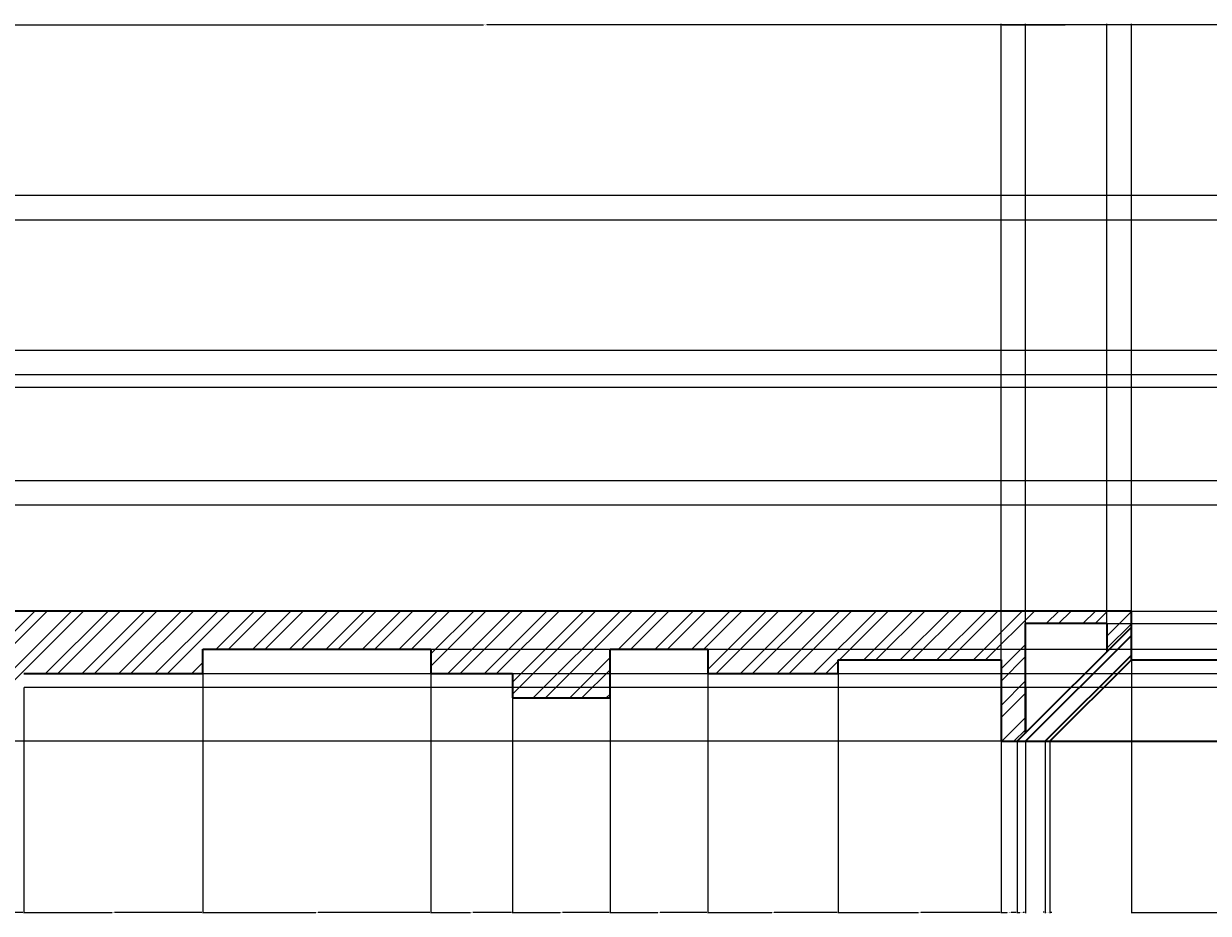
# Model space of a CAD drawing. Units: inches. Extents: x 2121 to 2815, y 1818 to 2233.
# Tile 4 of 6: x 2312 to 2530, y 2070 to 2233. Entities that reach past the tile are written whole.
import ezdxf

# ---------------------------------------------------------------- set-up
doc = ezdxf.new("R2010")
doc.units = ezdxf.units.IN
for name, color, linetype, lineweight in [('A-ANNO-DIMS', 2, 'Continuous', 18), ('A-COLS', 7, 'Continuous', 35), ('A-WALL', 7, 'Continuous', 35), ('A-WALL-PATT', 8, 'Continuous', 13)]:
    doc.layers.add(name, color=color, linetype=linetype, lineweight=lineweight)
doc.styles.get("Standard").update_dxf_attribs({"font": 'arial.ttf'})
doc.dimstyles.get("Standard").update_dxf_attribs({"dimtxt": 0.18, "dimasz": 0.18, "dimexe": 0.18, "dimexo": 0.0625, "dimgap": 0.09, "dimtad": 0, "dimtih": 1, "dimtoh": 1, "dimdec": 4, "dimzin": 0, "dimdsep": 46, "dimtxsty": 'Standard', "dimcen": 0.09, "dimadec": 0, "dimazin": 0, "dimtfac": 1, "dimtdec": 4, "dimtofl": 0, "dimtmove": 0, "dimatfit": 3, "dimfxl": 1, "dimtolj": 1, "dimtzin": 0, "dimarcsym": 0})

# ---------------------------------------------------------------- blocks, each defined once
blk = doc.blocks.new('*D10')
at = {"layer": 'A-ANNO-DIMS', "color": 0, "lineweight": -2, "transparency": 16777216}
for p, q in [((2152.83, 2129.87), (2152.83, 2233.48)), ((2153.01, 2233.3), (2396.54, 2233.3)), ((2640.65, 2233.3), (2397.13, 2233.3)), ((2640.83, 2129.87), (2640.83, 2233.48))]:
    blk.add_line(p, q, dxfattribs=at)
at = {"layer": 'A-ANNO-DIMS', "color": 0, "transparency": 16777216}
for points in [[(2153.01, 2233.33), (2153.01, 2233.27), (2152.83, 2233.3)], [(2640.65, 2233.33), (2640.65, 2233.27), (2640.83, 2233.3)]]:
    blk.add_solid(points, dxfattribs=at)
at = {"layer": 'Defpoints', "color": 0, "transparency": 16777216}
for p in [(2640.83, 2233.3), (2152.83, 2129.81), (2640.83, 2129.81)]:
    blk.add_point(p, dxfattribs=at)
at = {"layer": 'A-ANNO-DIMS', "color": 0, "transparency": 16777216, "insert": (2396.83, 2233.3), "char_height": 0.18, "attachment_point": 5}
blk.add_mtext('\\A1;488', dxfattribs=at)
blk = doc.blocks.new('*D17')
at = {"layer": 'A-ANNO-DIMS', "color": 0, "lineweight": -2, "transparency": 16777216}
for p, q in [((2287.83, 2111.25), (2287.83, 2069.63)), ((2311.83, 2111.25), (2311.83, 2069.63)), ((2288.01, 2069.81), (2299.61, 2069.81)), ((2311.65, 2069.81), (2300.05, 2069.81))]:
    blk.add_line(p, q, dxfattribs=at)
at = {"layer": 'A-ANNO-DIMS', "color": 0, "transparency": 16777216}
for points in [[(2288.01, 2069.84), (2288.01, 2069.78), (2287.83, 2069.81)], [(2311.65, 2069.84), (2311.65, 2069.78), (2311.83, 2069.81)]]:
    blk.add_solid(points, dxfattribs=at)
at = {"layer": 'Defpoints', "color": 0, "transparency": 16777216}
for p in [(2287.83, 2111.31), (2311.83, 2111.31), (2311.83, 2069.81)]:
    blk.add_point(p, dxfattribs=at)
at = {"layer": 'A-ANNO-DIMS', "color": 0, "transparency": 16777216, "insert": (2299.83, 2069.81), "char_height": 0.18, "attachment_point": 5}
blk.add_mtext('\\A1;24', dxfattribs=at)
blk = doc.blocks.new('*D18')
at = {"layer": 'A-ANNO-DIMS', "color": 0, "lineweight": -2, "transparency": 16777216}
for p, q in [((2344.83, 2113.75), (2344.83, 2069.63)), ((2311.83, 2111.25), (2311.83, 2069.63)), ((2312.01, 2069.81), (2328.11, 2069.81)), ((2344.65, 2069.81), (2328.55, 2069.81))]:
    blk.add_line(p, q, dxfattribs=at)
at = {"layer": 'A-ANNO-DIMS', "color": 0, "transparency": 16777216}
for points in [[(2312.01, 2069.84), (2312.01, 2069.78), (2311.83, 2069.81)], [(2344.65, 2069.84), (2344.65, 2069.78), (2344.83, 2069.81)]]:
    blk.add_solid(points, dxfattribs=at)
at = {"layer": 'Defpoints', "color": 0, "transparency": 16777216}
for p in [(2344.83, 2113.81), (2311.83, 2111.31), (2344.83, 2069.81)]:
    blk.add_point(p, dxfattribs=at)
at = {"layer": 'A-ANNO-DIMS', "color": 0, "transparency": 16777216, "insert": (2328.33, 2069.81), "char_height": 0.18, "attachment_point": 5}
blk.add_mtext('\\A1;33', dxfattribs=at)
blk = doc.blocks.new('*D19')
at = {"layer": 'A-ANNO-DIMS', "color": 0, "lineweight": -2, "transparency": 16777216}
for p, q in [((2344.83, 2113.75), (2344.83, 2069.63)), ((2386.83, 2113.75), (2386.83, 2069.63)), ((2345.01, 2069.81), (2365.61, 2069.81)), ((2386.65, 2069.81), (2366.05, 2069.81))]:
    blk.add_line(p, q, dxfattribs=at)
at = {"layer": 'A-ANNO-DIMS', "color": 0, "transparency": 16777216}
for points in [[(2345.01, 2069.84), (2345.01, 2069.78), (2344.83, 2069.81)], [(2386.65, 2069.84), (2386.65, 2069.78), (2386.83, 2069.81)]]:
    blk.add_solid(points, dxfattribs=at)
at = {"layer": 'Defpoints', "color": 0, "transparency": 16777216}
for p in [(2344.83, 2113.81), (2386.83, 2113.81), (2386.83, 2069.81)]:
    blk.add_point(p, dxfattribs=at)
at = {"layer": 'A-ANNO-DIMS', "color": 0, "transparency": 16777216, "insert": (2365.83, 2069.81), "char_height": 0.18, "attachment_point": 5}
blk.add_mtext('\\A1;42', dxfattribs=at)
blk = doc.blocks.new('*D20')
at = {"layer": 'A-ANNO-DIMS', "color": 0, "lineweight": -2, "transparency": 16777216}
for p, q in [((2386.83, 2113.75), (2386.83, 2069.63)), ((2401.83, 2109.25), (2401.83, 2069.63)), ((2387.01, 2069.81), (2394.12, 2069.81)), ((2401.65, 2069.81), (2394.54, 2069.81))]:
    blk.add_line(p, q, dxfattribs=at)
at = {"layer": 'A-ANNO-DIMS', "color": 0, "transparency": 16777216}
for points in [[(2387.01, 2069.84), (2387.01, 2069.78), (2386.83, 2069.81)], [(2401.65, 2069.84), (2401.65, 2069.78), (2401.83, 2069.81)]]:
    blk.add_solid(points, dxfattribs=at)
at = {"layer": 'Defpoints', "color": 0, "transparency": 16777216}
for p in [(2386.83, 2113.81), (2401.83, 2109.31), (2401.83, 2069.81)]:
    blk.add_point(p, dxfattribs=at)
at = {"layer": 'A-ANNO-DIMS', "color": 0, "transparency": 16777216, "insert": (2394.33, 2069.81), "char_height": 0.18, "attachment_point": 5}
blk.add_mtext('\\A1;15', dxfattribs=at)
blk = doc.blocks.new('*D21')
at = {"layer": 'A-ANNO-DIMS', "color": 0, "lineweight": -2, "transparency": 16777216}
for p, q in [((2401.83, 2109.25), (2401.83, 2069.63)), ((2419.83, 2109.25), (2419.83, 2069.63)), ((2402.01, 2069.81), (2410.62, 2069.81)), ((2419.65, 2069.81), (2411.04, 2069.81))]:
    blk.add_line(p, q, dxfattribs=at)
at = {"layer": 'A-ANNO-DIMS', "color": 0, "transparency": 16777216}
for points in [[(2402.01, 2069.84), (2402.01, 2069.78), (2401.83, 2069.81)], [(2419.65, 2069.84), (2419.65, 2069.78), (2419.83, 2069.81)]]:
    blk.add_solid(points, dxfattribs=at)
at = {"layer": 'Defpoints', "color": 0, "transparency": 16777216}
for p in [(2401.83, 2109.31), (2419.83, 2109.31), (2419.83, 2069.81)]:
    blk.add_point(p, dxfattribs=at)
at = {"layer": 'A-ANNO-DIMS', "color": 0, "transparency": 16777216, "insert": (2410.83, 2069.81), "char_height": 0.18, "attachment_point": 5}
blk.add_mtext('\\A1;18', dxfattribs=at)
blk = doc.blocks.new('*D22')
at = {"layer": 'A-ANNO-DIMS', "color": 0, "lineweight": -2, "transparency": 16777216}
for p, q in [((2437.83, 2113.75), (2437.83, 2069.63)), ((2419.83, 2109.25), (2419.83, 2069.63)), ((2420.01, 2069.81), (2428.62, 2069.81)), ((2437.65, 2069.81), (2429.04, 2069.81))]:
    blk.add_line(p, q, dxfattribs=at)
at = {"layer": 'A-ANNO-DIMS', "color": 0, "transparency": 16777216}
for points in [[(2420.01, 2069.84), (2420.01, 2069.78), (2419.83, 2069.81)], [(2437.65, 2069.84), (2437.65, 2069.78), (2437.83, 2069.81)]]:
    blk.add_solid(points, dxfattribs=at)
at = {"layer": 'Defpoints', "color": 0, "transparency": 16777216}
for p in [(2437.83, 2113.81), (2419.83, 2109.31), (2437.83, 2069.81)]:
    blk.add_point(p, dxfattribs=at)
at = {"layer": 'A-ANNO-DIMS', "color": 0, "transparency": 16777216, "insert": (2428.83, 2069.81), "char_height": 0.18, "attachment_point": 5}
blk.add_mtext('\\A1;18', dxfattribs=at)
blk = doc.blocks.new('*D23')
at = {"layer": 'A-ANNO-DIMS', "color": 0, "lineweight": -2, "transparency": 16777216}
for p, q in [((2437.83, 2113.75), (2437.83, 2069.63)), ((2461.83, 2113.75), (2461.83, 2069.63)), ((2438.01, 2069.81), (2449.61, 2069.81)), ((2461.65, 2069.81), (2450.05, 2069.81))]:
    blk.add_line(p, q, dxfattribs=at)
at = {"layer": 'A-ANNO-DIMS', "color": 0, "transparency": 16777216}
for points in [[(2438.01, 2069.84), (2438.01, 2069.78), (2437.83, 2069.81)], [(2461.65, 2069.84), (2461.65, 2069.78), (2461.83, 2069.81)]]:
    blk.add_solid(points, dxfattribs=at)
at = {"layer": 'Defpoints', "color": 0, "transparency": 16777216}
for p in [(2437.83, 2113.81), (2461.83, 2113.81), (2461.83, 2069.81)]:
    blk.add_point(p, dxfattribs=at)
at = {"layer": 'A-ANNO-DIMS', "color": 0, "transparency": 16777216, "insert": (2449.83, 2069.81), "char_height": 0.18, "attachment_point": 5}
blk.add_mtext('\\A1;24', dxfattribs=at)
blk = doc.blocks.new('*D24')
at = {"layer": 'A-ANNO-DIMS', "color": 0, "lineweight": -2, "transparency": 16777216}
for p, q in [((2461.83, 2113.75), (2461.83, 2069.63)), ((2491.83, 2101.25), (2491.83, 2069.63)), ((2462.01, 2069.81), (2476.61, 2069.81)), ((2491.65, 2069.81), (2477.05, 2069.81))]:
    blk.add_line(p, q, dxfattribs=at)
at = {"layer": 'A-ANNO-DIMS', "color": 0, "transparency": 16777216}
for points in [[(2462.01, 2069.84), (2462.01, 2069.78), (2461.83, 2069.81)], [(2491.65, 2069.84), (2491.65, 2069.78), (2491.83, 2069.81)]]:
    blk.add_solid(points, dxfattribs=at)
at = {"layer": 'Defpoints', "color": 0, "transparency": 16777216}
for p in [(2461.83, 2113.81), (2491.83, 2101.31), (2491.83, 2069.81)]:
    blk.add_point(p, dxfattribs=at)
at = {"layer": 'A-ANNO-DIMS', "color": 0, "transparency": 16777216, "insert": (2476.83, 2069.81), "char_height": 0.18, "attachment_point": 5}
blk.add_mtext('\\A1;30', dxfattribs=at)
blk = doc.blocks.new('*D25')
at = {"layer": 'A-ANNO-DIMS', "color": 0, "lineweight": -2, "transparency": 16777216}
for p, q in [((2491.83, 2101.37), (2491.83, 2233.48)), ((2492.01, 2233.3), (2503.61, 2233.3)), ((2515.65, 2233.3), (2504.05, 2233.3)), ((2515.83, 2125.37), (2515.83, 2233.48))]:
    blk.add_line(p, q, dxfattribs=at)
at = {"layer": 'A-ANNO-DIMS', "color": 0, "transparency": 16777216}
for points in [[(2492.01, 2233.33), (2492.01, 2233.27), (2491.83, 2233.3)], [(2515.65, 2233.33), (2515.65, 2233.27), (2515.83, 2233.3)]]:
    blk.add_solid(points, dxfattribs=at)
at = {"layer": 'Defpoints', "color": 0, "transparency": 16777216}
for p in [(2515.83, 2233.3), (2515.83, 2125.31), (2491.83, 2101.31)]:
    blk.add_point(p, dxfattribs=at)
at = {"layer": 'A-ANNO-DIMS', "color": 0, "transparency": 16777216, "insert": (2503.83, 2233.3), "char_height": 0.18, "attachment_point": 5}
blk.add_mtext('\\A1;24', dxfattribs=at)
blk = doc.blocks.new('*D26')
at = {"layer": 'A-ANNO-DIMS', "color": 0, "lineweight": -2, "transparency": 16777216}
for p, q in [((2515.83, 2116.25), (2515.83, 2069.63)), ((2619.83, 2108.3), (2619.83, 2069.63)), ((2516.01, 2069.81), (2567.55, 2069.81)), ((2619.65, 2069.81), (2568.11, 2069.81))]:
    blk.add_line(p, q, dxfattribs=at)
at = {"layer": 'A-ANNO-DIMS', "color": 0, "transparency": 16777216}
for points in [[(2516.01, 2069.84), (2516.01, 2069.78), (2515.83, 2069.81)], [(2619.65, 2069.84), (2619.65, 2069.78), (2619.83, 2069.81)]]:
    blk.add_solid(points, dxfattribs=at)
at = {"layer": 'Defpoints', "color": 0, "transparency": 16777216}
for p in [(2515.83, 2116.31), (2619.83, 2108.36), (2619.83, 2069.81)]:
    blk.add_point(p, dxfattribs=at)
at = {"layer": 'A-ANNO-DIMS', "color": 0, "transparency": 16777216, "insert": (2567.83, 2069.81), "char_height": 0.18, "attachment_point": 5}
blk.add_mtext('\\A1;104', dxfattribs=at)
blk = doc.blocks.new('*D32')
at = {"layer": 'A-ANNO-DIMS', "color": 0, "lineweight": -2, "transparency": 16777216}
for p, q in [((2311.9, 2113.81), (2814.07, 2113.81)), ((2813.89, 2113.63), (2813.89, 2112.74)), ((2813.89, 2111.49), (2813.89, 2112.38)), ((2311.9, 2111.31), (2814.07, 2111.31))]:
    blk.add_line(p, q, dxfattribs=at)
at = {"layer": 'A-ANNO-DIMS', "color": 0, "transparency": 16777216}
for points in [[(2813.86, 2113.63), (2813.92, 2113.63), (2813.89, 2113.81)], [(2813.86, 2111.49), (2813.92, 2111.49), (2813.89, 2111.31)]]:
    blk.add_solid(points, dxfattribs=at)
at = {"layer": 'Defpoints', "color": 0, "transparency": 16777216}
for p in [(2311.83, 2113.81), (2311.83, 2111.31), (2813.89, 2111.31)]:
    blk.add_point(p, dxfattribs=at)
at = {"layer": 'A-ANNO-DIMS', "color": 0, "transparency": 16777216, "insert": (2813.89, 2112.56), "char_height": 0.18, "attachment_point": 5}
blk.add_mtext('\\A1;2.5', dxfattribs=at)
blk = doc.blocks.new('*D33')
at = {"layer": 'A-ANNO-DIMS', "color": 0, "lineweight": -2, "transparency": 16777216}
for p, q in [((2386.9, 2118.31), (2814.07, 2118.31)), ((2813.89, 2118.13), (2813.89, 2116.24)), ((2813.89, 2113.99), (2813.89, 2115.88)), ((2386.9, 2113.81), (2814.07, 2113.81))]:
    blk.add_line(p, q, dxfattribs=at)
at = {"layer": 'A-ANNO-DIMS', "color": 0, "transparency": 16777216}
for points in [[(2813.86, 2118.13), (2813.92, 2118.13), (2813.89, 2118.31)], [(2813.86, 2113.99), (2813.92, 2113.99), (2813.89, 2113.81)]]:
    blk.add_solid(points, dxfattribs=at)
at = {"layer": 'Defpoints', "color": 0, "transparency": 16777216}
for p in [(2386.83, 2118.31), (2386.83, 2113.81), (2813.89, 2113.81)]:
    blk.add_point(p, dxfattribs=at)
at = {"layer": 'A-ANNO-DIMS', "color": 0, "transparency": 16777216, "insert": (2813.89, 2116.06), "char_height": 0.18, "attachment_point": 5}
blk.add_mtext('\\A1;4.5', dxfattribs=at)
blk = doc.blocks.new('*D34')
at = {"layer": 'A-ANNO-DIMS', "color": 0, "lineweight": -2, "transparency": 16777216}
for p, q in [((2515.9, 2116.31), (2814.07, 2116.31)), ((2813.89, 2116.13), (2813.89, 2108.99)), ((2813.89, 2101.49), (2813.89, 2108.63)), ((2500.9, 2101.31), (2814.07, 2101.31))]:
    blk.add_line(p, q, dxfattribs=at)
at = {"layer": 'A-ANNO-DIMS', "color": 0, "transparency": 16777216}
for points in [[(2813.86, 2116.13), (2813.92, 2116.13), (2813.89, 2116.31)], [(2813.86, 2101.49), (2813.92, 2101.49), (2813.89, 2101.31)]]:
    blk.add_solid(points, dxfattribs=at)
at = {"layer": 'Defpoints', "color": 0, "transparency": 16777216}
for p in [(2515.83, 2116.31), (2500.83, 2101.31), (2813.89, 2101.31)]:
    blk.add_point(p, dxfattribs=at)
at = {"layer": 'A-ANNO-DIMS', "color": 0, "transparency": 16777216, "insert": (2813.89, 2108.81), "char_height": 0.18, "attachment_point": 5}
blk.add_mtext('\\A1;15', dxfattribs=at)
blk = doc.blocks.new('*D36')
at = {"layer": 'A-ANNO-DIMS', "color": 0, "lineweight": -2, "transparency": 16777216}
for p, q in [((2515.77, 2125.31), (2121.16, 2125.31)), ((2121.34, 2125.13), (2121.34, 2113.49)), ((2121.34, 2101.49), (2121.34, 2113.13)), ((2491.77, 2101.31), (2121.16, 2101.31))]:
    blk.add_line(p, q, dxfattribs=at)
at = {"layer": 'A-ANNO-DIMS', "color": 0, "transparency": 16777216}
for points in [[(2121.31, 2125.13), (2121.37, 2125.13), (2121.34, 2125.31)], [(2121.31, 2101.49), (2121.37, 2101.49), (2121.34, 2101.31)]]:
    blk.add_solid(points, dxfattribs=at)
at = {"layer": 'Defpoints', "color": 0, "transparency": 16777216}
for p in [(2121.34, 2125.31), (2515.83, 2125.31), (2491.83, 2101.31)]:
    blk.add_point(p, dxfattribs=at)
at = {"layer": 'A-ANNO-DIMS', "color": 0, "transparency": 16777216, "insert": (2121.34, 2113.31), "char_height": 0.18, "attachment_point": 5}
blk.add_mtext('\\A1;24', dxfattribs=at)
blk = doc.blocks.new('*D37')
at = {"layer": 'A-ANNO-DIMS', "color": 0, "lineweight": -2, "transparency": 16777216}
for p, q in [((2491.83, 2116.37), (2491.83, 2233.48)), ((2492.01, 2233.3), (2493.82, 2233.3)), ((2496.15, 2233.3), (2494.34, 2233.3)), ((2496.33, 2123.06), (2496.33, 2233.48))]:
    blk.add_line(p, q, dxfattribs=at)
at = {"layer": 'A-ANNO-DIMS', "color": 0, "transparency": 16777216}
for points in [[(2492.01, 2233.33), (2492.01, 2233.27), (2491.83, 2233.3)], [(2496.15, 2233.33), (2496.15, 2233.27), (2496.33, 2233.3)]]:
    blk.add_solid(points, dxfattribs=at)
at = {"layer": 'Defpoints', "color": 0, "transparency": 16777216}
for p in [(2496.33, 2233.3), (2496.33, 2122.99), (2491.83, 2116.31)]:
    blk.add_point(p, dxfattribs=at)
at = {"layer": 'A-ANNO-DIMS', "color": 0, "transparency": 16777216, "insert": (2494.08, 2233.3), "char_height": 0.18, "attachment_point": 5}
blk.add_mtext('\\A1;4.5', dxfattribs=at)
blk = doc.blocks.new('*D38')
at = {"layer": 'A-ANNO-DIMS', "color": 0, "lineweight": -2, "transparency": 16777216}
for p, q in [((2496.33, 2123.06), (2496.33, 2233.48)), ((2496.51, 2233.3), (2503.62, 2233.3)), ((2511.15, 2233.3), (2504.04, 2233.3)), ((2511.33, 2123.06), (2511.33, 2233.48))]:
    blk.add_line(p, q, dxfattribs=at)
at = {"layer": 'A-ANNO-DIMS', "color": 0, "transparency": 16777216}
for points in [[(2496.51, 2233.33), (2496.51, 2233.27), (2496.33, 2233.3)], [(2511.15, 2233.33), (2511.15, 2233.27), (2511.33, 2233.3)]]:
    blk.add_solid(points, dxfattribs=at)
at = {"layer": 'Defpoints', "color": 0, "transparency": 16777216}
for p in [(2511.33, 2233.3), (2496.33, 2122.99), (2511.33, 2122.99)]:
    blk.add_point(p, dxfattribs=at)
at = {"layer": 'A-ANNO-DIMS', "color": 0, "transparency": 16777216, "insert": (2503.83, 2233.3), "char_height": 0.18, "attachment_point": 5}
blk.add_mtext('\\A1;15', dxfattribs=at)
blk = doc.blocks.new('*D39')
at = {"layer": 'A-ANNO-DIMS', "color": 0, "lineweight": -2, "transparency": 16777216}
for p, q in [((2515.9, 2125.31), (2814.07, 2125.31)), ((2813.89, 2125.13), (2813.89, 2124.33)), ((2511.4, 2122.99), (2814.07, 2122.99)), ((2813.89, 2123.17), (2813.89, 2123.97))]:
    blk.add_line(p, q, dxfattribs=at)
at = {"layer": 'A-ANNO-DIMS', "color": 0, "transparency": 16777216}
for points in [[(2813.86, 2125.13), (2813.92, 2125.13), (2813.89, 2125.31)], [(2813.86, 2123.17), (2813.92, 2123.17), (2813.89, 2122.99)]]:
    blk.add_solid(points, dxfattribs=at)
at = {"layer": 'Defpoints', "color": 0, "transparency": 16777216}
for p in [(2515.83, 2125.31), (2813.89, 2125.31), (2511.33, 2122.99)]:
    blk.add_point(p, dxfattribs=at)
at = {"layer": 'A-ANNO-DIMS', "color": 0, "transparency": 16777216, "insert": (2813.89, 2124.15), "char_height": 0.18, "attachment_point": 5}
blk.add_mtext('\\A1;2.314', dxfattribs=at)
blk = doc.blocks.new('*D40')
at = {"layer": 'A-ANNO-DIMS', "color": 0, "lineweight": -2, "transparency": 16777216}
for p, q in [((2491.83, 2101.25), (2491.83, 2069.63)), ((2494.81, 2101.25), (2494.81, 2069.63)), ((2492.01, 2069.81), (2492.95, 2069.81)), ((2494.63, 2069.81), (2493.7, 2069.81))]:
    blk.add_line(p, q, dxfattribs=at)
at = {"layer": 'A-ANNO-DIMS', "color": 0, "transparency": 16777216}
for points in [[(2492.01, 2069.84), (2492.01, 2069.78), (2491.83, 2069.81)], [(2494.63, 2069.84), (2494.63, 2069.78), (2494.81, 2069.81)]]:
    blk.add_solid(points, dxfattribs=at)
at = {"layer": 'Defpoints', "color": 0, "transparency": 16777216}
for p in [(2491.83, 2101.31), (2494.81, 2101.31), (2494.81, 2069.81)]:
    blk.add_point(p, dxfattribs=at)
at = {"layer": 'A-ANNO-DIMS', "color": 0, "transparency": 16777216, "insert": (2493.32, 2069.81), "char_height": 0.18, "attachment_point": 5}
blk.add_mtext('\\A1;2.981', dxfattribs=at)
blk = doc.blocks.new('*D41')
at = {"layer": 'A-ANNO-DIMS', "color": 0, "lineweight": -2, "transparency": 16777216}
for p, q in [((2494.81, 2101.25), (2494.81, 2069.63)), ((2496.33, 2101.25), (2496.33, 2069.63)), ((2494.99, 2069.81), (2495.26, 2069.81)), ((2496.15, 2069.81), (2495.89, 2069.81))]:
    blk.add_line(p, q, dxfattribs=at)
at = {"layer": 'A-ANNO-DIMS', "color": 0, "transparency": 16777216}
for points in [[(2494.99, 2069.84), (2494.99, 2069.78), (2494.81, 2069.81)], [(2496.15, 2069.84), (2496.15, 2069.78), (2496.33, 2069.81)]]:
    blk.add_solid(points, dxfattribs=at)
at = {"layer": 'Defpoints', "color": 0, "transparency": 16777216}
for p in [(2494.81, 2101.31), (2496.33, 2101.31), (2496.33, 2069.81)]:
    blk.add_point(p, dxfattribs=at)
at = {"layer": 'A-ANNO-DIMS', "color": 0, "transparency": 16777216, "insert": (2495.57, 2069.81), "char_height": 0.18, "attachment_point": 5}
blk.add_mtext('\\A1;1.52', dxfattribs=at)
blk = doc.blocks.new('*D42')
at = {"layer": 'A-ANNO-DIMS', "color": 0, "lineweight": -2, "transparency": 16777216}
for p, q in [((2499.935347, 2101.246525), (2499.935347, 2069.634025)), ((2500.832641, 2101.246525), (2500.832641, 2069.634025)), ((2499.755347, 2069.814025), (2499.575347, 2069.814025)), ((2501.012641, 2069.814025), (2501.192641, 2069.814025))]:
    blk.add_line(p, q, dxfattribs=at)
at = {"layer": 'A-ANNO-DIMS', "color": 0, "transparency": 16777216}
for points in [[(2499.755347, 2069.844025), (2499.755347, 2069.784025), (2499.935347, 2069.814025)], [(2501.012641, 2069.844025), (2501.012641, 2069.784025), (2500.832641, 2069.814025)]]:
    blk.add_solid(points, dxfattribs=at)
at = {"layer": 'Defpoints', "color": 0, "transparency": 16777216}
for p in [(2499.935347, 2101.309025), (2500.832641, 2101.309025), (2500.832641, 2069.814025)]:
    blk.add_point(p, dxfattribs=at)
at = {"layer": 'A-ANNO-DIMS', "color": 0, "transparency": 16777216, "insert": (2500.383994, 2069.814025), "char_height": 0.18, "attachment_point": 5}
blk.add_mtext('\\A1;0.90', dxfattribs=at)
blk = doc.blocks.new('*D86')
at = {"layer": 'A-ANNO-DIMS', "color": 0, "lineweight": -2, "transparency": 16777216}
for p, q in [((2760.77, 2144.81), (2121.16, 2144.81)), ((2121.34, 2144.63), (2121.34, 2123.24)), ((2121.34, 2101.49), (2121.34, 2122.88)), ((2760.77, 2101.31), (2121.16, 2101.31))]:
    blk.add_line(p, q, dxfattribs=at)
at = {"layer": 'A-ANNO-DIMS', "color": 0, "transparency": 16777216}
for points in [[(2121.31, 2144.63), (2121.37, 2144.63), (2121.34, 2144.81)], [(2121.31, 2101.49), (2121.37, 2101.49), (2121.34, 2101.31)]]:
    blk.add_solid(points, dxfattribs=at)
at = {"layer": 'Defpoints', "color": 0, "transparency": 16777216}
for p in [(2121.34, 2144.81), (2760.83, 2144.81), (2760.83, 2101.31)]:
    blk.add_point(p, dxfattribs=at)
at = {"layer": 'A-ANNO-DIMS', "color": 0, "transparency": 16777216, "insert": (2121.34, 2123.06), "char_height": 0.18, "attachment_point": 5}
blk.add_mtext('\\A1;43.5', dxfattribs=at)
blk = doc.blocks.new('*D88')
at = {"layer": 'A-ANNO-DIMS', "color": 0, "lineweight": -2, "transparency": 16777216}
for p, q in [((2760.77, 2197.31), (2121.16, 2197.31)), ((2121.34, 2197.13), (2121.34, 2185.49)), ((2121.34, 2173.49), (2121.34, 2185.13)), ((2760.77, 2173.31), (2121.16, 2173.31))]:
    blk.add_line(p, q, dxfattribs=at)
at = {"layer": 'A-ANNO-DIMS', "color": 0, "transparency": 16777216}
for points in [[(2121.31, 2197.13), (2121.37, 2197.13), (2121.34, 2197.31)], [(2121.31, 2173.49), (2121.37, 2173.49), (2121.34, 2173.31)]]:
    blk.add_solid(points, dxfattribs=at)
at = {"layer": 'Defpoints', "color": 0, "transparency": 16777216}
for p in [(2121.34, 2197.31), (2760.83, 2197.31), (2760.83, 2173.31)]:
    blk.add_point(p, dxfattribs=at)
at = {"layer": 'A-ANNO-DIMS', "color": 0, "transparency": 16777216, "insert": (2121.34, 2185.31), "char_height": 0.18, "attachment_point": 5}
blk.add_mtext('\\A1;24', dxfattribs=at)
blk = doc.blocks.new('*D89')
at = {"layer": 'A-ANNO-DIMS', "color": 0, "lineweight": -2, "transparency": 16777216}
for p, q in [((2756.07, 2201.81), (2121.16, 2201.81)), ((2121.34, 2201.63), (2121.34, 2199.74)), ((2121.34, 2197.49), (2121.34, 2199.38)), ((2760.77, 2197.31), (2121.16, 2197.31))]:
    blk.add_line(p, q, dxfattribs=at)
at = {"layer": 'A-ANNO-DIMS', "color": 0, "transparency": 16777216}
for points in [[(2121.31, 2201.63), (2121.37, 2201.63), (2121.34, 2201.81)], [(2121.31, 2197.49), (2121.37, 2197.49), (2121.34, 2197.31)]]:
    blk.add_solid(points, dxfattribs=at)
at = {"layer": 'Defpoints', "color": 0, "transparency": 16777216}
for p in [(2121.34, 2201.81), (2756.14, 2201.81), (2760.83, 2197.31)]:
    blk.add_point(p, dxfattribs=at)
at = {"layer": 'A-ANNO-DIMS', "color": 0, "transparency": 16777216, "insert": (2121.34, 2199.56), "char_height": 0.18, "attachment_point": 5}
blk.add_mtext('\\A1;4.5', dxfattribs=at)
blk = doc.blocks.new('*D90')
at = {"layer": 'A-ANNO-DIMS', "color": 0, "lineweight": -2, "transparency": 16777216}
for p, q in [((2760.77, 2168.81), (2121.16, 2168.81)), ((2121.34, 2168.63), (2121.34, 2159.24)), ((2121.34, 2149.49), (2121.34, 2158.88)), ((2760.77, 2149.31), (2121.16, 2149.31))]:
    blk.add_line(p, q, dxfattribs=at)
at = {"layer": 'A-ANNO-DIMS', "color": 0, "transparency": 16777216}
for points in [[(2121.31, 2168.63), (2121.37, 2168.63), (2121.34, 2168.81)], [(2121.31, 2149.49), (2121.37, 2149.49), (2121.34, 2149.31)]]:
    blk.add_solid(points, dxfattribs=at)
at = {"layer": 'Defpoints', "color": 0, "transparency": 16777216}
for p in [(2121.34, 2168.81), (2760.83, 2168.81), (2760.83, 2149.31)]:
    blk.add_point(p, dxfattribs=at)
at = {"layer": 'A-ANNO-DIMS', "color": 0, "transparency": 16777216, "insert": (2121.34, 2159.06), "char_height": 0.18, "attachment_point": 5}
blk.add_mtext('\\A1;19.5', dxfattribs=at)
blk = doc.blocks.new('*D91')
at = {"layer": 'A-ANNO-DIMS', "color": 0, "lineweight": -2, "transparency": 16777216}
for p, q in [((2760.77, 2149.31), (2121.16, 2149.31)), ((2121.34, 2149.13), (2121.34, 2147.24)), ((2121.34, 2144.99), (2121.34, 2146.88)), ((2760.77, 2144.81), (2121.16, 2144.81))]:
    blk.add_line(p, q, dxfattribs=at)
at = {"layer": 'A-ANNO-DIMS', "color": 0, "transparency": 16777216}
for points in [[(2121.31, 2149.13), (2121.37, 2149.13), (2121.34, 2149.31)], [(2121.31, 2144.99), (2121.37, 2144.99), (2121.34, 2144.81)]]:
    blk.add_solid(points, dxfattribs=at)
at = {"layer": 'Defpoints', "color": 0, "transparency": 16777216}
for p in [(2121.34, 2149.31), (2760.83, 2149.31), (2760.83, 2144.81)]:
    blk.add_point(p, dxfattribs=at)
at = {"layer": 'A-ANNO-DIMS', "color": 0, "transparency": 16777216, "insert": (2121.34, 2147.06), "char_height": 0.18, "attachment_point": 5}
blk.add_mtext('\\A1;4.5', dxfattribs=at)
blk = doc.blocks.new('*D97')
at = {"layer": 'A-ANNO-DIMS', "color": 0, "lineweight": -2, "transparency": 16777216}
for p, q in [((2765.42, 2168.81), (2121.16, 2168.81)), ((2121.34, 2168.63), (2121.34, 2167.83)), ((2765.42, 2166.48), (2121.16, 2166.48)), ((2121.34, 2166.66), (2121.34, 2167.46))]:
    blk.add_line(p, q, dxfattribs=at)
at = {"layer": 'A-ANNO-DIMS', "color": 0, "transparency": 16777216}
for points in [[(2121.31, 2168.63), (2121.37, 2168.63), (2121.34, 2168.81)], [(2121.31, 2166.66), (2121.37, 2166.66), (2121.34, 2166.48)]]:
    blk.add_solid(points, dxfattribs=at)
at = {"layer": 'Defpoints', "color": 0, "transparency": 16777216}
for p in [(2121.34, 2168.81), (2765.49, 2168.81), (2765.49, 2166.48)]:
    blk.add_point(p, dxfattribs=at)
at = {"layer": 'A-ANNO-DIMS', "color": 0, "transparency": 16777216, "insert": (2121.34, 2167.64), "char_height": 0.18, "attachment_point": 5}
blk.add_mtext('\\A1;2.33', dxfattribs=at)

msp = doc.modelspace()

# ---------------------------------------------------------------- hatches: boundary and pattern name
at = {"layer": 'A-WALL-PATT'}
h = msp.add_hatch(dxfattribs=at)
h.set_pattern_fill('ANSI32', color=256, scale=0.5)
h.paths.add_polyline_path([(2496.3326, 2122.9949), (2511.3326, 2122.9949), (2511.3326, 2117.8278), (2515.8326, 2122.3278), (2515.8326, 2125.309), (2157.3326, 2125.309), (2157.3326, 2129.809), (2152.8326, 2129.809), (2152.8326, 2125.309), (2152.8326, 2113.809), (2182.8326, 2113.809), (2182.8326, 2109.309), (2224.8326, 2109.309), (2224.8326, 2113.809), (2260.8326, 2113.809), (2260.8326, 2109.309), (2269.8326, 2109.309), (2269.8326, 2113.809), (2287.8326, 2113.809), (2287.8326, 2111.309), (2311.8326, 2111.309), (2311.8326, 2113.809), (2344.8326, 2113.809), (2344.8326, 2118.309), (2386.8326, 2118.309), (2386.8326, 2113.809), (2401.8326, 2113.809), (2401.8326, 2109.309), (2419.8326, 2109.309), (2419.8326, 2118.309), (2437.8326, 2118.309), (2437.8326, 2113.809), (2461.8326, 2113.809), (2461.8326, 2116.309), (2491.8326, 2116.309), (2491.8326, 2101.309), (2494.8138, 2101.309), (2496.3326, 2102.8278)])
h.paths.add_polyline_path([(2640.8326, 2129.809), (2628.8326, 2129.809), (2628.8326, 2125.309), (2619.8326, 2125.309), (2619.8326, 2108.3582), (2628.8326, 2101.309), (2640.8326, 2101.309)])

# ---------------------------------------------------------------- linework, layer by layer
at = {"layer": 'A-COLS'}
for p, q in [((2515.8326, 2116.309), (2515.8326, 2125.309)), ((2496.3326, 2102.8278), (2496.3326, 2122.9949)), ((2511.3326, 2122.9949), (2496.3326, 2122.9949)), ((2511.3326, 2122.9949), (2511.3326, 2117.8278)), ((2515.8326, 2122.3278), (2494.8138, 2101.309)), ((2515.8326, 2120.809), (2496.3326, 2101.309)), ((2515.8326, 2120.809), (2496.3326, 2101.309)), ((2491.8326, 2116.309), (2491.8326, 2101.309)), ((2515.8326, 2117.2063), (2499.9353, 2101.309)), ((2515.8326, 2116.309), (2500.8326, 2101.309)), ((2496.3326, 2111.2363), (2496.3326, 2111.2363)), ((2496.3326, 2111.2363), (2496.3326, 2102.8278)), ((2491.8326, 2101.309), (2500.8326, 2101.309))]:
    msp.add_line(p, q, dxfattribs=at)
at = {"layer": 'A-WALL'}
for p, q in [((2515.8326, 2125.309), (2157.3326, 2125.309)), ((2344.8326, 2113.809), (2344.8326, 2118.309)), ((2344.8326, 2118.309), (2386.8326, 2118.309)), ((2386.8326, 2118.309), (2386.8326, 2113.809)), ((2419.8326, 2109.309), (2419.8326, 2118.309)), ((2419.8326, 2118.309), (2437.8326, 2118.309)), ((2437.8326, 2118.309), (2437.8326, 2113.809)), ((2461.8326, 2113.809), (2461.8326, 2116.309)), ((2461.8326, 2116.309), (2491.8326, 2116.309)), ((2515.8326, 2116.309), (2619.8326, 2116.309)), ((2311.8326, 2113.809), (2344.8326, 2113.809)), ((2386.8326, 2113.809), (2401.8326, 2113.809)), ((2401.8326, 2113.809), (2401.8326, 2109.309)), ((2437.8326, 2113.809), (2461.8326, 2113.809)), ((2401.8326, 2109.309), (2419.8326, 2109.309)), ((2500.8326, 2101.309), (2778.8326, 2101.309))]:
    msp.add_line(p, q, dxfattribs=at)

# ---------------------------------------------------------------- dimensions: what is measured, and where the dimension line sits
at = {"layer": 'A-ANNO-DIMS'}
for base, p1, p2, override, picture, middle in [((2640.8326, 2233.304), (2152.8326, 2129.809), (2640.8326, 2129.809), {"dimdec": 0, "dimlfac": 1, "dimrnd": 0, "dimzin": 0, "dimdsep": 46, "dimlunit": 2}, '*D10', (2396.8326, 2233.304)), ((2515.8326, 2233.304), (2491.8326, 2101.309), (2515.8326, 2125.309), {"dimdec": 0, "dimlfac": 1, "dimrnd": 0, "dimzin": 0, "dimdsep": 46, "dimlunit": 2}, '*D25', (2503.8326, 2233.304)), ((2496.3326, 2233.304), (2491.8326, 2116.309), (2496.3326, 2122.9949), {"dimdec": 1, "dimlfac": 1, "dimrnd": 0, "dimzin": 0, "dimdsep": 46, "dimlunit": 2}, '*D37', (2494.0826, 2233.304)), ((2511.3326, 2233.304), (2496.3326, 2122.9949), (2511.3326, 2122.9949), {"dimdec": 0, "dimlfac": 1, "dimrnd": 0, "dimzin": 0, "dimdsep": 46, "dimlunit": 2}, '*D38', (2503.8326, 2233.304)), ((2619.8326, 2069.814), (2515.8326, 2116.309), (2619.8326, 2108.3582), {"dimdec": 0, "dimlfac": 1, "dimrnd": 0, "dimzin": 0, "dimdsep": 46, "dimlunit": 2}, '*D26', (2567.8326, 2069.814)), ((2344.8326, 2069.814), (2311.8326, 2111.309), (2344.8326, 2113.809), {"dimdec": 0, "dimlfac": 1, "dimrnd": 0, "dimzin": 0, "dimdsep": 46, "dimlunit": 2}, '*D18', (2328.3326, 2069.814)), ((2386.8326, 2069.814), (2344.8326, 2113.809), (2386.8326, 2113.809), {"dimdec": 0, "dimlfac": 1, "dimrnd": 0, "dimzin": 0, "dimdsep": 46, "dimlunit": 2}, '*D19', (2365.8326, 2069.814)), ((2401.8326, 2069.814), (2386.8326, 2113.809), (2401.8326, 2109.309), {"dimdec": 0, "dimlfac": 1, "dimrnd": 0, "dimzin": 0, "dimdsep": 46, "dimlunit": 2}, '*D20', (2394.3326, 2069.814)), ((2437.8326, 2069.814), (2419.8326, 2109.309), (2437.8326, 2113.809), {"dimdec": 0, "dimlfac": 1, "dimrnd": 0, "dimzin": 0, "dimdsep": 46, "dimlunit": 2}, '*D22', (2428.8326, 2069.814)), ((2461.8326, 2069.814), (2437.8326, 2113.809), (2461.8326, 2113.809), {"dimdec": 0, "dimlfac": 1, "dimrnd": 0, "dimzin": 0, "dimdsep": 46, "dimlunit": 2}, '*D23', (2449.8326, 2069.814)), ((2491.8326, 2069.814), (2461.8326, 2113.809), (2491.8326, 2101.309), {"dimdec": 0, "dimlfac": 1, "dimrnd": 0, "dimzin": 0, "dimdsep": 46, "dimlunit": 2}, '*D24', (2476.8326, 2069.814)), ((2311.8326, 2069.814), (2287.8326, 2111.309), (2311.8326, 2111.309), {"dimdec": 0, "dimlfac": 1, "dimrnd": 0, "dimzin": 0, "dimdsep": 46, "dimlunit": 2}, '*D17', (2299.8326, 2069.814)), ((2419.8326, 2069.814), (2401.8326, 2109.309), (2419.8326, 2109.309), {"dimdec": 0, "dimlfac": 1, "dimrnd": 0, "dimzin": 0, "dimdsep": 46, "dimlunit": 2}, '*D21', (2410.8326, 2069.814)), ((2494.8138, 2069.814), (2491.8326, 2101.309), (2494.8138, 2101.309), {"dimdec": 3, "dimlfac": 1, "dimrnd": 0, "dimzin": 0, "dimdsep": 46, "dimlunit": 2}, '*D40', (2493.3232, 2069.814)), ((2496.3326, 2069.814), (2494.8138, 2101.309), (2496.3326, 2101.309), {"dimdec": 2, "dimlfac": 1, "dimrnd": 0, "dimzin": 0, "dimdsep": 46, "dimlunit": 2}, '*D41', (2495.5732, 2069.814)), ((2500.8326, 2069.814), (2499.9353, 2101.309), (2500.8326, 2101.309), {"dimdec": 2, "dimlfac": 1, "dimrnd": 0, "dimzin": 0, "dimdsep": 46, "dimlunit": 2}, '*D42', (2500.384, 2069.814))]:
    dim = msp.add_linear_dim(base=base, p1=p1, p2=p2, dimstyle='Standard', override=override, dxfattribs=at)
    dim.commit()
    dim.dimension.update_dxf_attribs({"geometry": picture, "text_midpoint": middle})
for base, p1, p2, override, picture, middle in [((2121.3376, 2201.809), (2760.8326, 2197.309), (2756.1373, 2201.809), {"dimdec": 1, "dimlfac": 1, "dimrnd": 0, "dimzin": 0, "dimdsep": 46, "dimlunit": 2}, '*D89', (2121.3376, 2199.559)), ((2121.3376, 2197.309), (2760.8326, 2173.309), (2760.8326, 2197.309), {"dimdec": 0, "dimlfac": 1, "dimrnd": 0, "dimzin": 0, "dimdsep": 46, "dimlunit": 2}, '*D88', (2121.3376, 2185.309)), ((2121.3376, 2168.809), (2760.8326, 2149.309), (2760.8326, 2168.809), {"dimdec": 1, "dimlfac": 1, "dimrnd": 0, "dimzin": 0, "dimdsep": 46, "dimlunit": 2}, '*D90', (2121.3376, 2159.059)), ((2121.3376, 2168.809), (2765.4865, 2166.4788), (2765.4865, 2168.809), {"dimdec": 2, "dimlfac": 1, "dimrnd": 0, "dimzin": 0, "dimdsep": 46, "dimlunit": 2}, '*D97', (2121.3376, 2167.6439)), ((2121.3376, 2149.309), (2760.8326, 2144.809), (2760.8326, 2149.309), {"dimdec": 1, "dimlfac": 1, "dimrnd": 0, "dimzin": 0, "dimdsep": 46, "dimlunit": 2}, '*D91', (2121.3376, 2147.059)), ((2121.3376, 2144.809), (2760.8326, 2101.309), (2760.8326, 2144.809), {"dimdec": 1, "dimlfac": 1, "dimrnd": 0, "dimzin": 0, "dimdsep": 46, "dimlunit": 2}, '*D86', (2121.3376, 2123.059)), ((2121.3376, 2125.309), (2491.8326, 2101.309), (2515.8326, 2125.309), {"dimdec": 0, "dimlfac": 1, "dimrnd": 0, "dimzin": 0, "dimdsep": 46, "dimlunit": 2}, '*D36', (2121.3376, 2113.309)), ((2813.8872, 2125.309), (2511.3326, 2122.9949), (2515.8326, 2125.309), {"dimdec": 3, "dimlfac": 1, "dimrnd": 0, "dimzin": 0, "dimdsep": 46, "dimlunit": 2}, '*D39', (2813.8872, 2124.1519)), ((2813.8872, 2113.809), (2386.8326, 2118.309), (2386.8326, 2113.809), {"dimdec": 1, "dimlfac": 1, "dimrnd": 0, "dimzin": 0, "dimdsep": 46, "dimlunit": 2}, '*D33', (2813.8872, 2116.059)), ((2813.8872, 2101.309), (2515.8326, 2116.309), (2500.8326, 2101.309), {"dimdec": 0, "dimlfac": 1, "dimrnd": 0, "dimzin": 0, "dimdsep": 46, "dimlunit": 2}, '*D34', (2813.8872, 2108.809)), ((2813.8872, 2111.309), (2311.8326, 2113.809), (2311.8326, 2111.309), {"dimdec": 1, "dimlfac": 1, "dimrnd": 0, "dimzin": 0, "dimdsep": 46, "dimlunit": 2}, '*D32', (2813.8872, 2112.559))]:
    dim = msp.add_linear_dim(base=base, p1=p1, p2=p2, angle=90, dimstyle='Standard', override=override, dxfattribs=at)
    dim.commit()
    dim.dimension.update_dxf_attribs({"geometry": picture, "text_midpoint": middle})

doc.saveas('drawing.dxf')
